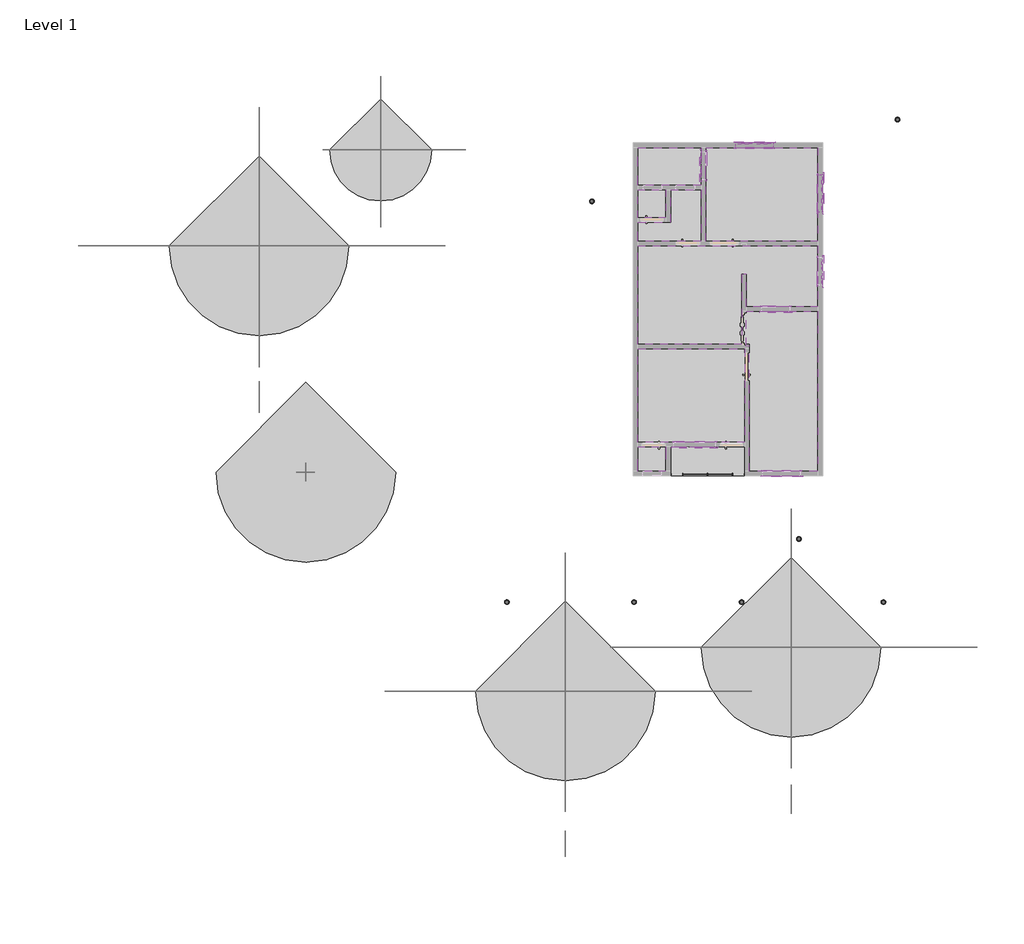
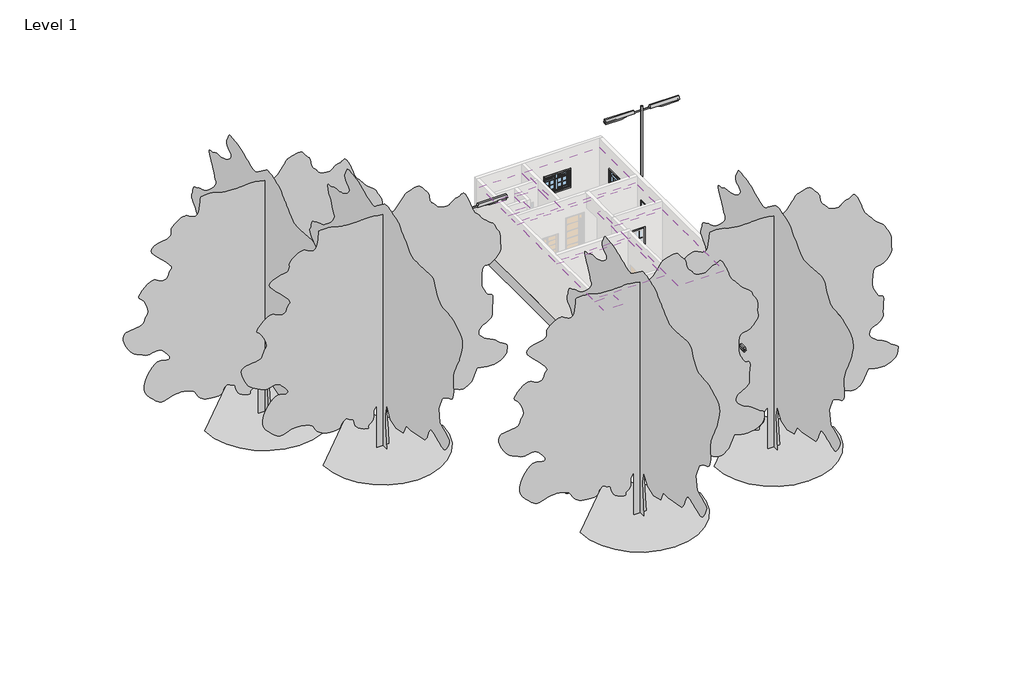
# One storey, part 2 of 2: 36 proxies, 8 coverings, 7 light fixtures, 5 geographic elements, 2 windows, 1 railing.
"""IFC4 building model written with IfcOpenShell, lengths in millimetres."""

from ifc_helpers import new_model, si_unit, point, frame, origin, place, context, project, spatial, polyline, ellipse_curve, trimmed, outline, extrude, transform, mapped, element, save
from ifc_brep_helpers import plane_surface, extruded_surface, advanced_brep
from components import m_muntin_pattern_2x2_m_muntin_pattern_2x2_ec2ff75e, m_muntin_pattern_2x2_m_muntin_pattern_2x2_6a19bea2, m_muntin_pattern_2x2_m_muntin_pattern_2x2_383df7b3, m_muntin_pattern_2x2_m_muntin_pattern_2x2_55460d9e, m_muntin_pattern_2x2_m_muntin_pattern_2x2_a9b7b7a9, m_muntin_pattern_2x2_m_muntin_pattern_2x2_c959817e, m_muntin_pattern_2x2_m_muntin_pattern_2x2_9259c5e2, m_trim_window_exterior_flat_with_sill_b1b88069, m_trim_window_exterior_flat_with_sill_8fa486dc, m_trim_window_exterior_flat_with_sill_2a9c44ae, m_trim_window_interior_flat_picture_frame_7d12f20c, m_trim_window_interior_flat_picture_frame_b6dd03a6, m_trim_window_interior_flat_picture_frame_c139440e, plinth_plinth_0a88a6c8, rpc_tree_deciduous_honey_locust_25_cc46a1f1, rpc_tree_deciduous_scarlet_oak_42_9b182cbb, light_fixture_105_street_light_dbl_105_street_light_dbl_4055396a, m_window_casement_double_awning_double_4_7efa9bbd

model = new_model("IFC4")

# Units and contexts
model_context = context("Model", 3, world=origin())
ifc_project = project(units=[si_unit("LENGTHUNIT", "METRE", prefix="MILLI")], contexts=[model_context])

# Site, building, storey
site = spatial("IfcSite", under=ifc_project)
building = spatial("IfcBuilding", under=site)
storey = spatial("IfcBuildingStorey", under=building, Name="Level 1", Elevation=0.0)

# Proxies
placement = place(None, origin())
m_muntin_pattern_2x2_m_muntin_pattern_2x2_shape = m_muntin_pattern_2x2_m_muntin_pattern_2x2_ec2ff75e(model_context)
element("IfcBuildingElementProxy", 1, Name="M_Muntin Pattern_2x2 : M_Muntin Pattern_2x2", ObjectType="M_Muntin Pattern_2x2 : M_Muntin Pattern_2x2", at=placement, inside=storey, context=model_context, shape_type="MappedRepresentation", body=[
    mapped(m_muntin_pattern_2x2_m_muntin_pattern_2x2_shape, transform((-20164.8088079, 6316.5492053, 1898.65), x_axis=(1.0, 0.0, 0.0), y_axis=(0.0, 1.0, 0.0), z_axis=(0.0, 0.0, 1.0))),
])
element("IfcBuildingElementProxy", 2, Name="M_Muntin Pattern_2x2 : M_Muntin Pattern_2x2", ObjectType="M_Muntin Pattern_2x2 : M_Muntin Pattern_2x2", at=placement, inside=storey, context=model_context, shape_type="MappedRepresentation", body=[
    mapped(m_muntin_pattern_2x2_m_muntin_pattern_2x2_shape, transform((-17648.6213079, 4984.6367053, 1898.65), x_axis=(0.0, -1.0, 0.0), y_axis=(1.0, 0.0, 0.0), z_axis=(0.0, 0.0, 1.0))),
])
element("IfcBuildingElementProxy", 3, Name="M_Muntin Pattern_2x2 : M_Muntin Pattern_2x2", ObjectType="M_Muntin Pattern_2x2 : M_Muntin Pattern_2x2", at=placement, inside=storey, context=model_context, shape_type="MappedRepresentation", body=[
    mapped(m_muntin_pattern_2x2_m_muntin_pattern_2x2_shape, transform((-18672.7572454, -4510.2007947, 1898.65), x_axis=(-1.0, 0.0, 0.0), y_axis=(0.0, -1.0, 0.0), z_axis=(0.0, 0.0, 1.0))),
])
m_muntin_pattern_2x2_m_muntin_pattern_2x2_2_shape = m_muntin_pattern_2x2_m_muntin_pattern_2x2_6a19bea2(model_context)
element("IfcBuildingElementProxy", 4, Name="M_Muntin Pattern_2x2 : M_Muntin Pattern_2x2", ObjectType="M_Muntin Pattern_2x2 : M_Muntin Pattern_2x2", at=placement, inside=storey, context=model_context, shape_type="MappedRepresentation", body=[
    mapped(m_muntin_pattern_2x2_m_muntin_pattern_2x2_2_shape, transform((-19558.3838079, 6316.5492053, 1898.65), x_axis=(-1.0, 0.0, 0.0), y_axis=(0.0, -1.0, 0.0), z_axis=(0.0, 0.0, 1.0))),
])
element("IfcBuildingElementProxy", 5, Name="M_Muntin Pattern_2x2 : M_Muntin Pattern_2x2", ObjectType="M_Muntin Pattern_2x2 : M_Muntin Pattern_2x2", at=placement, inside=storey, context=model_context, shape_type="MappedRepresentation", body=[
    mapped(m_muntin_pattern_2x2_m_muntin_pattern_2x2_2_shape, transform((-17648.6213079, 4378.2117053, 1898.65), x_axis=(0.0, 1.0, 0.0), y_axis=(-1.0, 0.0, 0.0), z_axis=(0.0, 0.0, 1.0))),
])
element("IfcBuildingElementProxy", 6, Name="M_Muntin Pattern_2x2 : M_Muntin Pattern_2x2", ObjectType="M_Muntin Pattern_2x2 : M_Muntin Pattern_2x2", at=placement, inside=storey, context=model_context, shape_type="MappedRepresentation", body=[
    mapped(m_muntin_pattern_2x2_m_muntin_pattern_2x2_2_shape, transform((-19279.1822454, -4510.2007947, 1898.65), x_axis=(1.0, 0.0, 0.0), y_axis=(0.0, 1.0, 0.0), z_axis=(0.0, 0.0, 1.0))),
])
m_muntin_pattern_2x2_m_muntin_pattern_2x2_3_shape = m_muntin_pattern_2x2_m_muntin_pattern_2x2_383df7b3(model_context)
element("IfcBuildingElementProxy", 7, Name="M_Muntin Pattern_2x2 : M_Muntin Pattern_2x2", ObjectType="M_Muntin Pattern_2x2 : M_Muntin Pattern_2x2", at=placement, inside=storey, context=model_context, shape_type="MappedRepresentation", body=[
    mapped(m_muntin_pattern_2x2_m_muntin_pattern_2x2_3_shape, transform((-19558.3838079, 6316.5492053, 2498.65), x_axis=(-1.0, 0.0, 0.0), y_axis=(0.0, -1.0, 0.0), z_axis=(0.0, 0.0, 1.0))),
])
element("IfcBuildingElementProxy", 8, Name="M_Muntin Pattern_2x2 : M_Muntin Pattern_2x2", ObjectType="M_Muntin Pattern_2x2 : M_Muntin Pattern_2x2", at=placement, inside=storey, context=model_context, shape_type="MappedRepresentation", body=[
    mapped(m_muntin_pattern_2x2_m_muntin_pattern_2x2_3_shape, transform((-20164.8088079, 6316.5492053, 2498.65), x_axis=(-1.0, 0.0, 0.0), y_axis=(0.0, -1.0, 0.0), z_axis=(0.0, 0.0, 1.0))),
])
element("IfcBuildingElementProxy", 9, Name="M_Muntin Pattern_2x2 : M_Muntin Pattern_2x2", ObjectType="M_Muntin Pattern_2x2 : M_Muntin Pattern_2x2", at=placement, inside=storey, context=model_context, shape_type="MappedRepresentation", body=[
    mapped(m_muntin_pattern_2x2_m_muntin_pattern_2x2_3_shape, transform((-17648.6213079, 4378.2117053, 2498.65), x_axis=(0.0, 1.0, 0.0), y_axis=(-1.0, 0.0, 0.0), z_axis=(0.0, 0.0, 1.0))),
])
element("IfcBuildingElementProxy", 10, Name="M_Muntin Pattern_2x2 : M_Muntin Pattern_2x2", ObjectType="M_Muntin Pattern_2x2 : M_Muntin Pattern_2x2", at=placement, inside=storey, context=model_context, shape_type="MappedRepresentation", body=[
    mapped(m_muntin_pattern_2x2_m_muntin_pattern_2x2_3_shape, transform((-17648.6213079, 4984.6367053, 2498.65), x_axis=(0.0, 1.0, 0.0), y_axis=(-1.0, 0.0, 0.0), z_axis=(0.0, 0.0, 1.0))),
])
element("IfcBuildingElementProxy", 11, Name="M_Muntin Pattern_2x2 : M_Muntin Pattern_2x2", ObjectType="M_Muntin Pattern_2x2 : M_Muntin Pattern_2x2", at=placement, inside=storey, context=model_context, shape_type="MappedRepresentation", body=[
    mapped(m_muntin_pattern_2x2_m_muntin_pattern_2x2_3_shape, transform((-19279.1822454, -4510.2007947, 2498.65), x_axis=(1.0, 0.0, 0.0), y_axis=(0.0, 1.0, 0.0), z_axis=(0.0, 0.0, 1.0))),
])
element("IfcBuildingElementProxy", 12, Name="M_Muntin Pattern_2x2 : M_Muntin Pattern_2x2", ObjectType="M_Muntin Pattern_2x2 : M_Muntin Pattern_2x2", at=placement, inside=storey, context=model_context, shape_type="MappedRepresentation", body=[
    mapped(m_muntin_pattern_2x2_m_muntin_pattern_2x2_3_shape, transform((-18672.7572454, -4510.2007947, 2498.65), x_axis=(1.0, 0.0, 0.0), y_axis=(0.0, 1.0, 0.0), z_axis=(0.0, 0.0, 1.0))),
])
m_muntin_pattern_2x2_m_muntin_pattern_2x2_4_shape = m_muntin_pattern_2x2_m_muntin_pattern_2x2_55460d9e(model_context)
element("IfcBuildingElementProxy", 13, Name="M_Muntin Pattern_2x2 : M_Muntin Pattern_2x2", ObjectType="M_Muntin Pattern_2x2 : M_Muntin Pattern_2x2", at=placement, inside=storey, context=model_context, shape_type="MappedRepresentation", body=[
    mapped(m_muntin_pattern_2x2_m_muntin_pattern_2x2_4_shape, transform((-18939.9533391, 849.1992053, 1898.65), x_axis=(-1.0, 0.0, 0.0), y_axis=(0.0, -1.0, 0.0), z_axis=(0.0, 0.0, 1.0))),
])
element("IfcBuildingElementProxy", 14, Name="M_Muntin Pattern_2x2 : M_Muntin Pattern_2x2", ObjectType="M_Muntin Pattern_2x2 : M_Muntin Pattern_2x2", at=placement, inside=storey, context=model_context, shape_type="MappedRepresentation", body=[
    mapped(m_muntin_pattern_2x2_m_muntin_pattern_2x2_4_shape, transform((-17648.6213079, 2366.8492053, 1898.65), x_axis=(0.0, -1.0, 0.0), y_axis=(1.0, 0.0, 0.0), z_axis=(0.0, 0.0, 1.0))),
])
element("IfcBuildingElementProxy", 15, Name="M_Muntin Pattern_2x2 : M_Muntin Pattern_2x2", ObjectType="M_Muntin Pattern_2x2 : M_Muntin Pattern_2x2", at=placement, inside=storey, context=model_context, shape_type="MappedRepresentation", body=[
    mapped(m_muntin_pattern_2x2_m_muntin_pattern_2x2_4_shape, transform((-21591.9713079, 5362.4617053, 1898.65), x_axis=(0.0, 1.0, 0.0), y_axis=(-1.0, 0.0, 0.0), z_axis=(0.0, 0.0, 1.0))),
])
m_muntin_pattern_2x2_m_muntin_pattern_2x2_5_shape = m_muntin_pattern_2x2_m_muntin_pattern_2x2_a9b7b7a9(model_context)
element("IfcBuildingElementProxy", 16, Name="M_Muntin Pattern_2x2 : M_Muntin Pattern_2x2", ObjectType="M_Muntin Pattern_2x2 : M_Muntin Pattern_2x2", at=placement, inside=storey, context=model_context, shape_type="MappedRepresentation", body=[
    mapped(m_muntin_pattern_2x2_m_muntin_pattern_2x2_5_shape, transform((-19393.9783391, 849.1992053, 1898.65), x_axis=(1.0, 0.0, 0.0), y_axis=(0.0, 1.0, 0.0), z_axis=(0.0, 0.0, 1.0))),
])
element("IfcBuildingElementProxy", 17, Name="M_Muntin Pattern_2x2 : M_Muntin Pattern_2x2", ObjectType="M_Muntin Pattern_2x2 : M_Muntin Pattern_2x2", at=placement, inside=storey, context=model_context, shape_type="MappedRepresentation", body=[
    mapped(m_muntin_pattern_2x2_m_muntin_pattern_2x2_5_shape, transform((-17648.6213079, 1912.8242053, 1898.65), x_axis=(0.0, 1.0, 0.0), y_axis=(-1.0, 0.0, 0.0), z_axis=(0.0, 0.0, 1.0))),
])
element("IfcBuildingElementProxy", 18, Name="M_Muntin Pattern_2x2 : M_Muntin Pattern_2x2", ObjectType="M_Muntin Pattern_2x2 : M_Muntin Pattern_2x2", at=placement, inside=storey, context=model_context, shape_type="MappedRepresentation", body=[
    mapped(m_muntin_pattern_2x2_m_muntin_pattern_2x2_5_shape, transform((-21591.9713079, 5816.4867053, 1898.65), x_axis=(0.0, -1.0, 0.0), y_axis=(1.0, 0.0, 0.0), z_axis=(0.0, 0.0, 1.0))),
])
m_muntin_pattern_2x2_m_muntin_pattern_2x2_6_shape = m_muntin_pattern_2x2_m_muntin_pattern_2x2_c959817e(model_context)
element("IfcBuildingElementProxy", 19, Name="M_Muntin Pattern_2x2 : M_Muntin Pattern_2x2", ObjectType="M_Muntin Pattern_2x2 : M_Muntin Pattern_2x2", at=placement, inside=storey, context=model_context, shape_type="MappedRepresentation", body=[
    mapped(m_muntin_pattern_2x2_m_muntin_pattern_2x2_6_shape, transform((-21364.4296412, -3570.4007947, 1898.65), x_axis=(-1.0, 0.0, 0.0), y_axis=(0.0, -1.0, 0.0), z_axis=(0.0, 0.0, 1.0))),
])
m_muntin_pattern_2x2_m_muntin_pattern_2x2_7_shape = m_muntin_pattern_2x2_m_muntin_pattern_2x2_9259c5e2(model_context)
element("IfcBuildingElementProxy", 20, Name="M_Muntin Pattern_2x2 : M_Muntin Pattern_2x2", ObjectType="M_Muntin Pattern_2x2 : M_Muntin Pattern_2x2", at=placement, inside=storey, context=model_context, shape_type="MappedRepresentation", body=[
    mapped(m_muntin_pattern_2x2_m_muntin_pattern_2x2_7_shape, transform((-22257.6629746, -3570.4007947, 1898.65), x_axis=(1.0, 0.0, 0.0), y_axis=(0.0, 1.0, 0.0), z_axis=(0.0, 0.0, 1.0))),
])
element("IfcBuildingElementProxy", 21, Name="M_Muntin Pattern_2x2 : M_Muntin Pattern_2x2", ObjectType="M_Muntin Pattern_2x2 : M_Muntin Pattern_2x2", at=placement, inside=storey, context=model_context, shape_type="MappedRepresentation", body=[
    mapped(m_muntin_pattern_2x2_m_muntin_pattern_2x2_7_shape, transform((-21811.0463079, -3570.4007947, 1898.65), x_axis=(1.0, 0.0, 0.0), y_axis=(0.0, 1.0, 0.0), z_axis=(0.0, 0.0, 1.0))),
])
m_trim_window_exterior_flat_with_sill_shape = m_trim_window_exterior_flat_with_sill_b1b88069(model_context)
element("IfcBuildingElementProxy", 22, Name="M_Trim-Window-Exterior-Flat : with Sill", ObjectType="M_Trim-Window-Exterior-Flat : with Sill", at=placement, inside=storey, context=model_context, shape_type="MappedRepresentation", body=[
    mapped(m_trim_window_exterior_flat_with_sill_shape, transform((-19861.5963079, 6326.0742053, 2728.8), x_axis=(-1.0, 0.0, 0.0), y_axis=(0.0, 0.0, 1.0), z_axis=(0.0, 1.0, 0.0))),
])
element("IfcBuildingElementProxy", 23, Name="M_Trim-Window-Exterior-Flat : with Sill", ObjectType="M_Trim-Window-Exterior-Flat : with Sill", at=placement, inside=storey, context=model_context, shape_type="MappedRepresentation", body=[
    mapped(m_trim_window_exterior_flat_with_sill_shape, transform((-17639.0963079, 4681.4242053, 2728.8), x_axis=(0.0, 1.0, 0.0), y_axis=(0.0, 0.0, 1.0), z_axis=(1.0, 0.0, 0.0))),
])
element("IfcBuildingElementProxy", 24, Name="M_Trim-Window-Exterior-Flat : with Sill", ObjectType="M_Trim-Window-Exterior-Flat : with Sill", at=placement, inside=storey, context=model_context, shape_type="MappedRepresentation", body=[
    mapped(m_trim_window_exterior_flat_with_sill_shape, transform((-18975.9697454, -4519.7257947, 2728.8), x_axis=(1.0, 0.0, 0.0), y_axis=(0.0, 0.0, 1.0), z_axis=(0.0, -1.0, 0.0))),
])
m_trim_window_exterior_flat_with_sill_2_shape = m_trim_window_exterior_flat_with_sill_8fa486dc(model_context)
element("IfcBuildingElementProxy", 25, Name="M_Trim-Window-Exterior-Flat : with Sill", ObjectType="M_Trim-Window-Exterior-Flat : with Sill", at=placement, inside=storey, context=model_context, shape_type="MappedRepresentation", body=[
    mapped(m_trim_window_exterior_flat_with_sill_2_shape, transform((-19166.9658391, 839.6742053, 2728.8), x_axis=(1.0, 0.0, 0.0), y_axis=(0.0, 0.0, 1.0), z_axis=(0.0, -1.0, 0.0))),
])
element("IfcBuildingElementProxy", 26, Name="M_Trim-Window-Exterior-Flat : with Sill", ObjectType="M_Trim-Window-Exterior-Flat : with Sill", at=placement, inside=storey, context=model_context, shape_type="MappedRepresentation", body=[
    mapped(m_trim_window_exterior_flat_with_sill_2_shape, transform((-17639.0963079, 2139.8367053, 2728.8), x_axis=(0.0, 1.0, 0.0), y_axis=(0.0, 0.0, 1.0), z_axis=(1.0, 0.0, 0.0))),
])
element("IfcBuildingElementProxy", 27, Name="M_Trim-Window-Exterior-Flat : with Sill", ObjectType="M_Trim-Window-Exterior-Flat : with Sill", at=placement, inside=storey, context=model_context, shape_type="MappedRepresentation", body=[
    mapped(m_trim_window_exterior_flat_with_sill_2_shape, transform((-21601.4963079, 5589.4742053, 2728.8), x_axis=(0.0, -1.0, 0.0), y_axis=(0.0, 0.0, 1.0), z_axis=(-1.0, 0.0, 0.0))),
])
m_trim_window_exterior_flat_with_sill_3_shape = m_trim_window_exterior_flat_with_sill_2a9c44ae(model_context)
element("IfcBuildingElementProxy", 28, Name="M_Trim-Window-Exterior-Flat : with Sill", ObjectType="M_Trim-Window-Exterior-Flat : with Sill", at=placement, inside=storey, context=model_context, shape_type="MappedRepresentation", body=[
    mapped(m_trim_window_exterior_flat_with_sill_3_shape, transform((-21811.0463079, -3579.9257947, 2628.8), x_axis=(1.0, 0.0, 0.0), y_axis=(0.0, 0.0, 1.0), z_axis=(0.0, -1.0, 0.0))),
])
m_trim_window_interior_flat_picture_frame_shape = m_trim_window_interior_flat_picture_frame_7d12f20c(model_context)
element("IfcBuildingElementProxy", 29, Name="M_Trim-Window-Interior-Flat : Picture Frame", ObjectType="M_Trim-Window-Interior-Flat : Picture Frame", at=placement, inside=storey, context=model_context, shape_type="MappedRepresentation", body=[
    mapped(m_trim_window_interior_flat_picture_frame_shape, transform((-19861.5963079, 6173.6742053, 2728.8), x_axis=(1.0, 0.0, 0.0), y_axis=(0.0, 0.0, 1.0), z_axis=(0.0, -1.0, 0.0))),
])
element("IfcBuildingElementProxy", 30, Name="M_Trim-Window-Interior-Flat : Picture Frame", ObjectType="M_Trim-Window-Interior-Flat : Picture Frame", at=placement, inside=storey, context=model_context, shape_type="MappedRepresentation", body=[
    mapped(m_trim_window_interior_flat_picture_frame_shape, transform((-17791.4963079, 4681.4242053, 2728.8), x_axis=(0.0, -1.0, 0.0), y_axis=(0.0, 0.0, 1.0), z_axis=(-1.0, 0.0, 0.0))),
])
element("IfcBuildingElementProxy", 31, Name="M_Trim-Window-Interior-Flat : Picture Frame", ObjectType="M_Trim-Window-Interior-Flat : Picture Frame", at=placement, inside=storey, context=model_context, shape_type="MappedRepresentation", body=[
    mapped(m_trim_window_interior_flat_picture_frame_shape, transform((-18975.9697454, -4367.3257947, 2728.8), x_axis=(-1.0, 0.0, 0.0), y_axis=(0.0, 0.0, 1.0), z_axis=(0.0, 1.0, 0.0))),
])
m_trim_window_interior_flat_picture_frame_2_shape = m_trim_window_interior_flat_picture_frame_b6dd03a6(model_context)
element("IfcBuildingElementProxy", 32, Name="M_Trim-Window-Interior-Flat : Picture Frame", ObjectType="M_Trim-Window-Interior-Flat : Picture Frame", at=placement, inside=storey, context=model_context, shape_type="MappedRepresentation", body=[
    mapped(m_trim_window_interior_flat_picture_frame_2_shape, transform((-19166.9658391, 992.0742053, 2728.8), x_axis=(-1.0, 0.0, 0.0), y_axis=(0.0, 0.0, 1.0), z_axis=(0.0, 1.0, 0.0))),
])
element("IfcBuildingElementProxy", 33, Name="M_Trim-Window-Interior-Flat : Picture Frame", ObjectType="M_Trim-Window-Interior-Flat : Picture Frame", at=placement, inside=storey, context=model_context, shape_type="MappedRepresentation", body=[
    mapped(m_trim_window_interior_flat_picture_frame_2_shape, transform((-17791.4963079, 2139.8367053, 2728.8), x_axis=(0.0, -1.0, 0.0), y_axis=(0.0, 0.0, 1.0), z_axis=(-1.0, 0.0, 0.0))),
])
element("IfcBuildingElementProxy", 34, Name="M_Trim-Window-Interior-Flat : Picture Frame", ObjectType="M_Trim-Window-Interior-Flat : Picture Frame", at=placement, inside=storey, context=model_context, shape_type="MappedRepresentation", body=[
    mapped(m_trim_window_interior_flat_picture_frame_2_shape, transform((-21449.0963079, 5589.4742053, 2728.8), x_axis=(0.0, 1.0, 0.0), y_axis=(0.0, 0.0, 1.0), z_axis=(1.0, 0.0, 0.0))),
])
m_trim_window_interior_flat_picture_frame_3_shape = m_trim_window_interior_flat_picture_frame_c139440e(model_context)
element("IfcBuildingElementProxy", 35, Name="M_Trim-Window-Interior-Flat : Picture Frame", ObjectType="M_Trim-Window-Interior-Flat : Picture Frame", at=placement, inside=storey, context=model_context, shape_type="MappedRepresentation", body=[
    mapped(m_trim_window_interior_flat_picture_frame_3_shape, transform((-21811.0463079, -3427.5257947, 2628.8), x_axis=(-1.0, 0.0, 0.0), y_axis=(0.0, 0.0, 1.0), z_axis=(0.0, 1.0, 0.0))),
])
plinth_plinth_shape = plinth_plinth_0a88a6c8(model_context)
element("IfcBuildingElementProxy", 36, Name="PLINTH : PLINTH", ObjectType="PLINTH : PLINTH", at=placement, inside=storey, context=model_context, shape_type="MappedRepresentation", body=[
    mapped(plinth_plinth_shape, transform((0.0, 0.0, 0.0), x_axis=(1.0, 0.0, 0.0), y_axis=(0.0, 1.0, 0.0), z_axis=(0.0, 0.0, 1.0))),
])

# Coverings
element("IfcCovering", 37, ObjectType="2' x 4' ACT System", at=placement, inside=storey, context=model_context, shape_type="SweptSolid", body=[
    extrude(outline(polyline([(-23658.8963079, 6173.6742053), (-21601.4963079, 6173.6742053), (-21601.4963079, 4954.4742053), (-23658.8963079, 4954.4742053), (-23658.8963079, 6173.6742053)])), frame((0.0, 0.0, 3352.8), z_axis=(0.0, 0.0, 1.0), x_axis=(1.0, 0.0, 0.0)), (0.0, 0.0, 1.0), 57.15),
])
element("IfcCovering", 38, ObjectType="2' x 4' ACT System", at=placement, inside=storey, context=model_context, shape_type="SweptSolid", body=[
    extrude(outline(polyline([(-21449.0963079, 3125.6742053), (-21449.0963079, 6173.6742053), (-17791.4963079, 6173.6742053), (-17791.4963079, 3125.6742053), (-21449.0963079, 3125.6742053)])), frame((0.0, 0.0, 3352.8), z_axis=(0.0, 0.0, 1.0), x_axis=(1.0, 0.0, 0.0)), (0.0, 0.0, 1.0), 57.15),
])
element("IfcCovering", 39, ObjectType="2' x 4' ACT System", at=placement, inside=storey, context=model_context, shape_type="SweptSolid", body=[
    extrude(outline(polyline([(-21601.4963079, 3125.6742053), (-23658.8963079, 3125.6742053), (-23658.8963079, 3735.2742053), (-22592.0963079, 3735.2742053), (-22592.0963079, 4802.0742053), (-21601.4963079, 4802.0742053), (-21601.4963079, 3125.6742053)])), frame((0.0, 0.0, 3352.8), z_axis=(0.0, 0.0, 1.0), x_axis=(1.0, 0.0, 0.0)), (0.0, 0.0, 1.0), 57.15),
])
element("IfcCovering", 40, ObjectType="2' x 4' ACT System", at=placement, inside=storey, context=model_context, shape_type="SweptSolid", body=[
    extrude(outline(polyline([(-22744.4963079, 3887.6742053), (-23658.8963079, 3887.6742053), (-23658.8963079, 4802.0742053), (-22744.4963079, 4802.0742053), (-22744.4963079, 3887.6742053)])), frame((0.0, 0.0, 3352.8), z_axis=(0.0, 0.0, 1.0), x_axis=(1.0, 0.0, 0.0)), (0.0, 0.0, 1.0), 57.15),
])
element("IfcCovering", 41, ObjectType="2' x 4' ACT System", at=placement, inside=storey, context=model_context, shape_type="SweptSolid", body=[
    extrude(outline(polyline([(-17791.4963079, 2973.2742053), (-17791.4963079, 992.0742053), (-20128.2963079, 992.0742053), (-20128.2963079, 2050.5574639), (-20280.6963079, 2050.5574639), (-20280.6963079, 915.8742053), (-20280.6963079, -227.1257947), (-23658.8963079, -227.1257947), (-23658.8963079, 2973.2742053), (-17791.4963079, 2973.2742053)])), frame((0.0, 0.0, 3352.8), z_axis=(0.0, 0.0, 1.0), x_axis=(1.0, 0.0, 0.0)), (0.0, 0.0, 1.0), 57.15),
])
element("IfcCovering", 42, ObjectType="2' x 4' ACT System", at=placement, inside=storey, context=model_context, shape_type="SweptSolid", body=[
    extrude(outline(polyline([(-20179.0963079, -3427.5257947), (-23658.8963079, -3427.5257947), (-23658.8963079, -379.5257947), (-20179.0963079, -379.5257947), (-20179.0963079, -3427.5257947)])), frame((0.0, 0.0, 3352.8), z_axis=(0.0, 0.0, 1.0), x_axis=(1.0, 0.0, 0.0)), (0.0, 0.0, 1.0), 57.15),
])
element("IfcCovering", 43, ObjectType="2' x 4' ACT System", at=placement, inside=storey, context=model_context, shape_type="SweptSolid", body=[
    extrude(outline(polyline([(-17791.4963079, 839.6742053), (-17791.4963079, -4367.3257947), (-20026.6963079, -4367.3257947), (-20026.6963079, -303.3257947), (-20128.2963079, -303.3257947), (-20128.2963079, 839.6742053), (-17791.4963079, 839.6742053)])), frame((0.0, 0.0, 3352.8), z_axis=(0.0, 0.0, 1.0), x_axis=(1.0, 0.0, 0.0)), (0.0, 0.0, 1.0), 57.15),
])
element("IfcCovering", 44, ObjectType="2' x 4' ACT System", at=placement, inside=storey, context=model_context, shape_type="SweptSolid", body=[
    extrude(outline(polyline([(-22744.4963079, -4367.3257947), (-23658.8963079, -4367.3257947), (-23658.8963079, -3579.9257947), (-22744.4963079, -3579.9257947), (-22744.4963079, -4367.3257947)])), frame((0.0, 0.0, 3352.8), z_axis=(0.0, 0.0, 1.0), x_axis=(1.0, 0.0, 0.0)), (0.0, 0.0, 1.0), 57.15),
])

# Geographic elements
rpc_tree_deciduous_honey_locust_25_shape = rpc_tree_deciduous_honey_locust_25_cc46a1f1(model_context)
element("IfcGeographicElement", 45, ObjectType="RPC Tree - Deciduous : Honey Locust - 25'", at=placement, inside=storey, context=model_context, shape_type="MappedRepresentation", body=[
    mapped(rpc_tree_deciduous_honey_locust_25_shape, transform((-32040.8963079, 6097.4742053, -1981.2), x_axis=(1.0, 0.0, 0.0), y_axis=(0.0, 1.0, 0.0), z_axis=(0.0, 0.0, 1.0))),
])
rpc_tree_deciduous_scarlet_oak_42_shape = rpc_tree_deciduous_scarlet_oak_42_9b182cbb(model_context)
element("IfcGeographicElement", 46, ObjectType="RPC Tree - Deciduous : Scarlet Oak - 42'", at=placement, inside=storey, context=model_context, shape_type="MappedRepresentation", body=[
    mapped(rpc_tree_deciduous_scarlet_oak_42_shape, transform((-36003.2963079, 2973.2742053, -1981.2), x_axis=(1.0, 0.0, 0.0), y_axis=(0.0, 1.0, 0.0), z_axis=(0.0, 0.0, 1.0))),
])
element("IfcGeographicElement", 47, ObjectType="RPC Tree - Deciduous : Scarlet Oak - 42'", at=placement, inside=storey, context=model_context, shape_type="MappedRepresentation", body=[
    mapped(rpc_tree_deciduous_scarlet_oak_42_shape, transform((-26020.9810533, -11530.6777483, -1928.1661647), x_axis=(1.0, 0.0, 0.0), y_axis=(0.0, 1.0, 0.0), z_axis=(0.0, 0.0, 1.0))),
])
element("IfcGeographicElement", 48, ObjectType="RPC Tree - Deciduous : Scarlet Oak - 42'", at=placement, inside=storey, context=model_context, shape_type="MappedRepresentation", body=[
    mapped(rpc_tree_deciduous_scarlet_oak_42_shape, transform((-18667.7963079, -10107.7142603, -1960.082478), x_axis=(1.0, 0.0, 0.0), y_axis=(0.0, 1.0, 0.0), z_axis=(0.0, 0.0, 1.0))),
])
element("IfcGeographicElement", 49, ObjectType="RPC Tree - Deciduous : Scarlet Oak - 42'", at=placement, inside=storey, context=model_context, shape_type="MappedRepresentation", body=[
    mapped(rpc_tree_deciduous_scarlet_oak_42_shape, transform((-34477.6655413, -4403.0556437, 186.7246553), x_axis=(1.0, 0.0, 0.0), y_axis=(0.0, 1.0, 0.0), z_axis=(0.0, 0.0, 1.0))),
])

# Light fixtures
light_fixture_105_street_light_dbl_105_street_light_dbl_shape = light_fixture_105_street_light_dbl_105_street_light_dbl_4055396a(model_context)
element("IfcLightFixture", 50, ObjectType="105_Street Light - Dbl : 105_Street Light - Dbl", at=placement, inside=storey, context=model_context, shape_type="MappedRepresentation", body=[
    mapped(light_fixture_105_street_light_dbl_105_street_light_dbl_shape, transform((-25157.4963079, 4377.509477, -1981.2), x_axis=(0.0, 1.0, 0.0), y_axis=(-1.0, 0.0, 0.0), z_axis=(0.0, 0.0, 1.0))),
])
element("IfcLightFixture", 51, ObjectType="105_Street Light - Dbl : 105_Street Light - Dbl", at=placement, inside=storey, context=model_context, shape_type="MappedRepresentation", body=[
    mapped(light_fixture_105_street_light_dbl_105_street_light_dbl_shape, transform((-15200.6963079, 7044.509477, -1981.2), x_axis=(0.0, 1.0, 0.0), y_axis=(-1.0, 0.0, 0.0), z_axis=(0.0, 0.0, 1.0))),
])
element("IfcLightFixture", 52, ObjectType="105_Street Light - Dbl : 105_Street Light - Dbl", at=placement, inside=storey, context=model_context, shape_type="MappedRepresentation", body=[
    mapped(light_fixture_105_street_light_dbl_105_street_light_dbl_shape, transform((-18457.3610362, -6577.1257947, -1981.2), x_axis=(1.0, 0.0, 0.0), y_axis=(0.0, 1.0, 0.0), z_axis=(0.0, 0.0, 1.0))),
])
element("IfcLightFixture", 53, ObjectType="105_Street Light - Dbl : 105_Street Light - Dbl", at=placement, inside=storey, context=model_context, shape_type="MappedRepresentation", body=[
    mapped(light_fixture_105_street_light_dbl_105_street_light_dbl_shape, transform((-27969.6610362, -8634.5257947, -1981.2), x_axis=(1.0, 0.0, 0.0), y_axis=(0.0, 1.0, 0.0), z_axis=(0.0, 0.0, 1.0))),
])
element("IfcLightFixture", 54, ObjectType="105_Street Light - Dbl : 105_Street Light - Dbl", at=placement, inside=storey, context=model_context, shape_type="MappedRepresentation", body=[
    mapped(light_fixture_105_street_light_dbl_105_street_light_dbl_shape, transform((-23829.4610362, -8634.5257947, -1981.2), x_axis=(1.0, 0.0, 0.0), y_axis=(0.0, 1.0, 0.0), z_axis=(0.0, 0.0, 1.0))),
])
element("IfcLightFixture", 55, ObjectType="105_Street Light - Dbl : 105_Street Light - Dbl", at=placement, inside=storey, context=model_context, shape_type="MappedRepresentation", body=[
    mapped(light_fixture_105_street_light_dbl_105_street_light_dbl_shape, transform((-20324.2610362, -8634.5257947, -1981.2), x_axis=(1.0, 0.0, 0.0), y_axis=(0.0, 1.0, 0.0), z_axis=(0.0, 0.0, 1.0))),
])
element("IfcLightFixture", 56, ObjectType="105_Street Light - Dbl : 105_Street Light - Dbl", at=placement, inside=storey, context=model_context, shape_type="MappedRepresentation", body=[
    mapped(light_fixture_105_street_light_dbl_105_street_light_dbl_shape, transform((-15701.4610362, -8634.5257947, -1981.2), x_axis=(1.0, 0.0, 0.0), y_axis=(0.0, 1.0, 0.0), z_axis=(0.0, 0.0, 1.0))),
])

# Railing
element("IfcRailing", 57, ObjectType="Glass Panel - Bottom Fill", at=placement, inside=storey, context=model_context, shape_type="SolidModel", body=[
    advanced_brep(
    [(-22592.0963079, -4430.8257947, 1828.8), (-22592.0963079, -4507.0257947, 1828.8), (-20179.0963079, -4430.8257947, 1828.8), (-20179.0963079, -4507.0257947, 1828.8)],
    [
        (0, 1, ellipse_curve(frame((-22592.0963079, -4468.9257947, 1828.8), z_axis=(-1.0, 0.0, 0.0), x_axis=(0.0, -1.0, 0.0)), 38.1, 28.575)),
        (1, 0, ellipse_curve(frame((-22592.0963079, -4468.9257947, 1828.8), z_axis=(-1.0, 0.0, 0.0), x_axis=(0.0, -1.0, 0.0)), 38.1, 28.575)),
        (2, 3, ellipse_curve(frame((-20179.0963079, -4468.9257947, 1828.8), z_axis=(1.0, 0.0, 0.0), x_axis=(0.0, -1.0, 0.0)), 38.1, 28.575)),
        (3, 2, ellipse_curve(frame((-20179.0963079, -4468.9257947, 1828.8), z_axis=(1.0, 0.0, 0.0), x_axis=(0.0, -1.0, 0.0)), 38.1, 28.575)),
        (0, 2),
        (3, 1),
    ],
    [
        plane_surface(frame((-22592.0963079, -4468.9257947, 1828.8), z_axis=(-1.0, 0.0, 0.0), x_axis=(0.0, 1.0, 0.0))),
        plane_surface(frame((-20179.0963079, -4468.9257947, 1828.8), z_axis=(1.0, 0.0, 0.0), x_axis=(0.0, 1.0, 0.0))),
        extruded_surface(trimmed(ellipse_curve(frame((-20179.0963079, -4468.9257947, 1828.8), z_axis=(-1.0, 0.0, 0.0), x_axis=(0.0, -1.0, 0.0)), 38.1, 28.575), [point((-20179.0963079, -4430.8257947, 1828.8))], [point((-20179.0963079, -4507.0257947, 1828.8))], True, "CARTESIAN"), (-2413.0, 0.0, 0.0), 2413.0),
        extruded_surface(trimmed(ellipse_curve(frame((-20179.0963079, -4468.9257947, 1828.8), z_axis=(-1.0, 0.0, 0.0), x_axis=(0.0, -1.0, 0.0)), 38.1, 28.575), [point((-20179.0963079, -4507.0257947, 1828.8))], [point((-20179.0963079, -4430.8257947, 1828.8))], True, "CARTESIAN"), (-2413.0, 0.0, 0.0), 2413.0),
    ],
    [
        (0, [[1, 2]]),
        (1, [[3, 4]]),
        (2, [[-1, 5, -4, 6]]),
        (3, [[-2, -6, -3, -5]]),
    ],
),
    extrude(outline(polyline([(-22592.0963079, -4481.6257947), (-22592.0963079, -4456.2257947), (-20179.0963079, -4456.2257947), (-20179.0963079, -4481.6257947), (-22592.0963079, -4481.6257947)])), frame((0.0, 0.0, 1511.3), z_axis=(0.0, 0.0, 1.0), x_axis=(1.0, 0.0, 0.0)), (0.0, 0.0, 1.0), 25.4),
    extrude(outline(polyline([(-22592.0963079, -4481.6257947), (-22592.0963079, -4456.2257947), (-20179.0963079, -4456.2257947), (-20179.0963079, -4481.6257947), (-22592.0963079, -4481.6257947)])), frame((0.0, 0.0, 1308.1), z_axis=(0.0, 0.0, 1.0), x_axis=(1.0, 0.0, 0.0)), (0.0, 0.0, 1.0), 25.4),
    extrude(outline(polyline([(-20579.1463079, -4494.3257947), (-20579.1463079, -4443.5257947), (-20566.4463079, -4443.5257947), (-20566.4463079, -4494.3257947), (-20579.1463079, -4494.3257947)])), frame((0.0, 0.0, 609.6), z_axis=(0.0, 0.0, 1.0), x_axis=(1.0, 0.0, 0.0)), (0.0, 0.0, 1.0), 1190.625),
    extrude(outline(polyline([(-21385.5963079, -4462.3906377), (-20572.7963079, -4462.3906377), (-20572.7963079, -4468.7406377), (-21385.5963079, -4468.7406377), (-21385.5963079, -4462.3906377)])), frame((0.0, 0.0, 711.2), z_axis=(0.0, 0.0, 1.0), x_axis=(1.0, 0.0, 0.0)), (0.0, 0.0, 1.0), 711.2),
    extrude(outline(polyline([(-21391.9463079, -4494.3257947), (-21391.9463079, -4443.5257947), (-21379.2463079, -4443.5257947), (-21379.2463079, -4494.3257947), (-21391.9463079, -4494.3257947)])), frame((0.0, 0.0, 609.6), z_axis=(0.0, 0.0, 1.0), x_axis=(1.0, 0.0, 0.0)), (0.0, 0.0, 1.0), 1190.625),
    extrude(outline(polyline([(-22198.3963079, -4462.3906377), (-21385.5963079, -4462.3906377), (-21385.5963079, -4468.7406377), (-22198.3963079, -4468.7406377), (-22198.3963079, -4462.3906377)])), frame((0.0, 0.0, 711.2), z_axis=(0.0, 0.0, 1.0), x_axis=(1.0, 0.0, 0.0)), (0.0, 0.0, 1.0), 711.2),
    extrude(outline(polyline([(-22204.7463079, -4494.3257947), (-22204.7463079, -4443.5257947), (-22192.0463079, -4443.5257947), (-22192.0463079, -4494.3257947), (-22204.7463079, -4494.3257947)])), frame((0.0, 0.0, 609.6), z_axis=(0.0, 0.0, 1.0), x_axis=(1.0, 0.0, 0.0)), (0.0, 0.0, 1.0), 1190.625),
    extrude(outline(polyline([(-20191.7963079, -4478.4507947), (-20191.7963079, -4459.4007947), (-20172.7463079, -4459.4007947), (-20172.7463079, -4478.4507947), (-20191.7963079, -4478.4507947)])), frame((0.0, 0.0, 609.6), z_axis=(0.0, 0.0, 1.0), x_axis=(1.0, 0.0, 0.0)), (0.0, 0.0, 1.0), 1190.625),
    extrude(outline(polyline([(-22598.4463079, -4478.4507947), (-22598.4463079, -4459.4007947), (-22579.3963079, -4459.4007947), (-22579.3963079, -4478.4507947), (-22598.4463079, -4478.4507947)])), frame((0.0, 0.0, 609.6), z_axis=(0.0, 0.0, 1.0), x_axis=(1.0, 0.0, 0.0)), (0.0, 0.0, 1.0), 1190.625),
])

# Windows
m_window_casement_double_awning_double_4_shape = m_window_casement_double_awning_double_4_7efa9bbd(model_context)
element("IfcWindow", 58, ObjectType="M_Window-Casement-Double-Awning-Double : 4'", at=placement, inside=storey, context=model_context, shape_type="MappedRepresentation", body=[
    mapped(m_window_casement_double_awning_double_4_shape, transform((-19861.5963079, 6249.8742053, 928.8), x_axis=(1.0, 0.0, 0.0), y_axis=(0.0, 1.0, 0.0), z_axis=(0.0, 0.0, 1.0))),
])
element("IfcWindow", 59, ObjectType="M_Window-Casement-Double-Awning-Double : 4'", at=placement, inside=storey, context=model_context, shape_type="MappedRepresentation", body=[
    mapped(m_window_casement_double_awning_double_4_shape, transform((-17715.2963079, 4681.4242053, 928.8), x_axis=(0.0, -1.0, 0.0), y_axis=(1.0, 0.0, 0.0), z_axis=(0.0, 0.0, 1.0))),
])

save(model, "model.ifc")

# Revit data of these elements
# Type "M_Muntin Pattern_2x2 : M_Muntin Pattern_2x2"
#   Width [instance default] = 3' - 11.24409"
#   Thickness = 0' - 0 1/2"
#   Height [instance default] = 3' - 11.24409"
#   Distance = 0' - 0 3/4"
#   Interior Material [instance default] = none
#   Exterior Material [instance default] = none
#   Default Elevation = 0
# Type "M_Trim-Window-Exterior-Flat : with Sill"
#   Trim Width = 0' - 2.3622"
#   Trim Thickness_Picture Frame = 0' - 1.1811"
#   Trim Thickness_with Sill = 0' - 0 3/4"
#   Sill Thickness = 0' - 1.1811"
#   Opening Width [instance default] = 1' - 11.62205"
#   Opening Height [instance default] = 2' - 11.43307"
#   Default Elevation = 3' - 11.24409"
#   Sill = yes
#   Picture Frame = no
#   Trim Material [instance default] = none
# Type "M_Trim-Window-Interior-Flat : Picture Frame"
#   Trim Thickness_Picture Frame = 0' - 1.1811"
#   Trim Width = 0' - 2.3622"
#   Trim Thickness_with Sill = 0' - 0.7874"
#   Sill Thickness = 0' - 1.1811"
#   Opening Width [instance default] = 1' - 11.62205"
#   Opening Height [instance default] = 2' - 11.43307"
#   Default Elevation = 3' - 11.24409"
#   Sill = no
#   Picture Frame = yes
#   Trim Material [instance default] = none
# Type "2' x 4' ACT System"
#   Assembly Code = "C3030210"
#   built-in parameter 1002203 = 1 (stored number, unit not read)
#   built-in parameter 1002202 = 1 (stored number, unit not read)
#   Layers, outside or top first: 0' - 1 5/8" "Default" (function 1); 0' - 0 5/8" "Acoustic Ceiling Tile 24 x 48" (function 5)
# Type "RPC Tree - Deciduous : Honey Locust - 25'"
#   built-in parameter 1005198 = "{2, 15},{39, RPC-16-G2VH-N100-5X50-0000-ST1L-LVER-AU},{1, 0},{1, 0},{2, 13},{1, 8},{5, Color},{1, 0},{1, 0},{3, 0.8},{3, 0.8},{3, 0.8},{1, 8},{7, BBoxMin},{1, 0},{1, 0},{1, 0},{1, 0},{1, 0},{1, 8},{7, BBoxMax},{1, 0},{1, 0},{1, 0},{1, 0},{1, 0},{2, 11},{9, RPCTypeId},{1, 0},{1, 0},{39, RPC-16-G2VH-N100-5X50-0000-ST1L-LVER-AU},{1, 6},{14, RPCPlantHeight},{1, 0},{1, 0},{2, 25},{2, 11},{7, keyword},{1, 0},{1, 0},{34, :RPCs:Trees [General]:Geometry:RPC},{2, 11},{8, category},{1, 0},{1, 0},{15, Trees [General]},{2, 11},{12, LocalizedUID},{1, 0},{1, 0},{12, Honey-Locust},{2, 14},{6, Height},{1, 0},{1, 0},{2, 25},{1, 2},{16, Cast Reflections},{1, 0},{1, 0},{1, 0},{1, 2},{12, Cast Shadows},{1, 0},{1, 0},{1, 1},{1, 2},{9, Lock View},{1, 0},{1, 0},{1, 0},{1, 4},{5, ViewC},{1, 0},{1, 0},{1, 0},{21, assetlibrary_base.fbx},{1, 5},"
#   built-in parameter 1005195 = "RPC-16-G2VH-N100-5X50-0000-ST1L-LVER-AU"
#   Type Comments = "Honey Locust"
#   Assembly Code = "G2050500"
#   Height = 25' - 0"
#   Default Elevation = 0
# Type "RPC Tree - Deciduous : Scarlet Oak - 42'"
#   built-in parameter 1005198 = "{2, 15},{39, RPC-16-G0FB-J5PX-0LX6-U000-ST1L-LVER-AU},{1, 0},{1, 0},{2, 13},{1, 8},{5, Color},{1, 0},{1, 0},{3, 0.8},{3, 0.8},{3, 0.8},{1, 8},{7, BBoxMin},{1, 0},{1, 0},{1, 0},{1, 0},{1, 0},{1, 8},{7, BBoxMax},{1, 0},{1, 0},{1, 0},{1, 0},{1, 0},{2, 11},{9, RPCTypeId},{1, 0},{1, 0},{39, RPC-16-G0FB-J5PX-0LX6-U000-ST1L-LVER-AU},{1, 6},{14, RPCPlantHeight},{1, 0},{1, 0},{2, 42},{2, 11},{7, keyword},{1, 0},{1, 0},{34, :RPCs:Trees [General]:Geometry:RPC},{2, 11},{8, category},{1, 0},{1, 0},{15, Trees [General]},{2, 11},{12, LocalizedUID},{1, 0},{1, 0},{11, Scarlet_Oak},{2, 14},{6, Height},{1, 0},{1, 0},{2, 42},{1, 2},{16, Cast Reflections},{1, 0},{1, 0},{1, 0},{1, 2},{12, Cast Shadows},{1, 0},{1, 0},{1, 1},{1, 2},{9, Lock View},{1, 0},{1, 0},{1, 0},{1, 4},{5, ViewC},{1, 0},{1, 0},{1, 0},{21, assetlibrary_base.fbx},{1, 5},"
#   built-in parameter 1005195 = "RPC-16-G0FB-J5PX-0LX6-U000-ST1L-LVER-AU"
#   Type Comments = "Scarlet Oak"
#   Assembly Code = "G2050500"
#   Height = 42' - 0"
#   Default Elevation = 0
# Type "105_Street Light - Dbl : 105_Street Light - Dbl"
#   Keynote = "V"
#   Wattage = 500 W
#   built-in parameter 1150110 = 1 (stored number, unit not read)
#   built-in parameter 1114217 = 2.64 (stored number, unit not read)
#   built-in parameter 1150109 = 1 (stored number, unit not read)
#   built-in parameter 1150113 = 1 (stored number, unit not read)
#   built-in parameter 1150105 = 5910.3 (stored number, unit not read)
#   Lumens = 74271 lm
#   built-in parameter 1150115 = 1 (stored number, unit not read)
#   Light Source Symbol Size = 2' - 0"
#   built-in parameter 1150112 = 1 (stored number, unit not read)
#   built-in parameter 1150114 = 1 (stored number, unit not read)
#   built-in parameter 1150107 = 6000 (stored number, unit not read)
#   built-in parameter 1150106 = 59.103 (stored number, unit not read)
#   Height = 19' - 8.22047"
#   built-in parameter 1150104 = 13.8 (stored number, unit not read)
#   Base Height = 4' - 11.05512"
#   built-in parameter 1114218 = 1 (stored number, unit not read)
#   built-in parameter 1150133 = 10 (stored number, unit not read)
#   Arm Length = 5' - 10.86614"
#   built-in parameter 1150134 = 5
#   Color Filter = 16777215
#   Material Lamp Post = Paint - Black Matte
#   Material Lamp Glazing = Glass
#   Dimming Lamp Color Temperature Shift = (empty or 0)
#   Default Elevation = 0
# Type "Glass Panel - Bottom Fill"
#   Assembly Code = "C2010400"
#   built-in parameter 1008612 = 0.0416667 (stored number, unit not read)
#   built-in parameter 1008611 = 0.0416667 (stored number, unit not read)
#   built-in parameter 1008609 = 0.333333 (stored number, unit not read)
#   built-in parameter 1008604 = 0.166667 (stored number, unit not read)
#   built-in parameter 1008603 = 0.166667 (stored number, unit not read)
#   Railing Height = 4' - 0"
#   built-in parameter 1008630 = 2
#   built-in parameter 1008610 = 2
#   built-in parameter 1008618 = Baluster - Square : 3/4"
# Type "M_Window-Casement-Double-Awning-Double : 4'"
#   Type Mark = "11"
#   Fire Rating = "0.5h"
#   Assembly Code = "B2020100"
#   Analytic Construction = "Double glazing - domestic"
#   Window Inset [instance default] = 0' - 0"
#   Wall Thickness [instance default] = 0' - 5.90551"
#   Interior Wall Closure [instance default] = 0' - 2.15551"
#   Half Width = 2' - 0"
#   Visual Light Transmittance = 0.81
#   Transom Height = 0' - 11.81102"
#   Thermal Resistance (R) = 1.8146 (h·ft²·°F)/BTU
#   Solar Heat Gain Coefficient = 0.76
#   Rough Width = 4' - 0.59055"
#   Rough Height = 3' - 0.02362"
#   Open Window Height = 1' - 11.62205"
#   Frame Extension [instance default] = 0' - 0 1/4"
#   Height = 2' - 11.43307"
#   Heat Transfer Coefficient (U) = 0.5511 BTU/(h·ft²·°F)
#   Exterior Wall Closure [instance default] = 0' - 1.25197"
#   Extension Jamb [instance default] = 0' - 2.15551"
#   Default Sill Height = 2' - 11.43307"
#   Width = 4' - 0"
#   Top Muntin Visibility = yes
#   Bottom Muntin Visibility = yes
#   Interior Trim Visibility [instance default] = yes
#   Exterior Trim Visibility [instance default] = yes
#   Extension Jamb Visibility [instance default] = yes
#   Interior Trim Material = Wood - Stained
#   Muntin Pattern = M_Muntin Pattern_2x2 : M_Muntin Pattern_2x2
#   Interior Trim = M_Trim-Window-Interior-Flat : Picture Frame
#   Interior Frame Material = Wood - Stained
#   Glass Panel Material = Glass
#   Exterior Trim Material = Clad - White
#   Exterior Trim = M_Trim-Window-Exterior-Flat : with Sill
#   Exterior Frame Material = Clad - White
#   Wall Closure = (empty or 0)
# Elements 1, 2, 3, 4, 5, 6 (IfcBuildingElementProxy, "M_Muntin Pattern_2x2 : M_Muntin Pattern_2x2")
#   Width = 1' - 6 5/8"
#   Height = 1' - 6.12205"
#   Interior Material = Wood - Stained
#   Exterior Material = Clad - White
#   Phase Created = New Construction
#   Materials on its faces: "Clad - White", "Wood - Stained"
# Elements 7, 8, 9, 10, 11, 12 (IfcBuildingElementProxy, "M_Muntin Pattern_2x2 : M_Muntin Pattern_2x2")
#   Width = 1' - 6 5/8"
#   Height = 0' - 6.31102"
#   Interior Material = Wood - Stained
#   Exterior Material = Clad - White
#   Phase Created = New Construction
#   Materials on its faces: "Clad - White", "Wood - Stained"
# Elements 13, 14, 15, 16, 17, 18 (IfcBuildingElementProxy, "M_Muntin Pattern_2x2 : M_Muntin Pattern_2x2")
#   Width = 1' - 0 5/8"
#   Height = 2' - 5.93307"
#   Interior Material = Wood - Stained
#   Exterior Material = Clad - White
#   Phase Created = New Construction
#   Materials on its faces: "Clad - White", "Wood - Stained"
# Elements 19, 20, 21 (IfcBuildingElementProxy, "M_Muntin Pattern_2x2 : M_Muntin Pattern_2x2")
#   Width = 1' - 0.33333"
#   Height = 2' - 1.99606"
#   Interior Material = Wood - Stained
#   Exterior Material = Clad - White
#   Phase Created = New Construction
#   Materials on its faces: "Clad - White", "Wood - Stained"
# Elements 22, 23, 24 (IfcBuildingElementProxy, "M_Trim-Window-Exterior-Flat : with Sill")
#   Opening Width = 4' - 0"
#   Opening Height = 2' - 11.43307"
#   Trim Material = Clad - White
#   Phase Created = New Construction
#   Materials on its faces: "Clad - White"
# Elements 25, 26, 27 (IfcBuildingElementProxy, "M_Trim-Window-Exterior-Flat : with Sill")
#   Opening Width = 3' - 0"
#   Opening Height = 2' - 11.43307"
#   Trim Material = Clad - White
#   Phase Created = New Construction
#   Materials on its faces: "Clad - White"
# Element 28 (IfcBuildingElementProxy, "M_Trim-Window-Exterior-Flat : with Sill")
#   Opening Width = 4' - 5"
#   Opening Height = 2' - 7.49606"
#   Trim Material = Clad - White
#   Phase Created = New Construction
#   Materials on its faces: "Clad - White"
# Elements 29, 30, 31 (IfcBuildingElementProxy, "M_Trim-Window-Interior-Flat : Picture Frame")
#   Opening Width = 4' - 0"
#   Opening Height = 2' - 11.43307"
#   Trim Material = Wood - Stained
#   Phase Created = New Construction
#   Materials on its faces: "Wood - Stained"
# Elements 32, 33, 34 (IfcBuildingElementProxy, "M_Trim-Window-Interior-Flat : Picture Frame")
#   Opening Width = 3' - 0"
#   Opening Height = 2' - 11.43307"
#   Trim Material = Wood - Stained
#   Phase Created = New Construction
#   Materials on its faces: "Wood - Stained"
# Element 35 (IfcBuildingElementProxy, "M_Trim-Window-Interior-Flat : Picture Frame")
#   Opening Width = 4' - 5"
#   Opening Height = 2' - 7.49606"
#   Trim Material = Wood - Stained
#   Phase Created = New Construction
#   Materials on its faces: "Wood - Stained"
# Element 36 (IfcBuildingElementProxy, "PLINTH : PLINTH")
#   Phase Created = New Construction
# Elements 37, 38, 39, 40, 41, 42, 43, 44 (IfcCovering, "2' x 4' ACT System")
#   Height Offset From Level = 11' - 0"
#   Phase Created = New Construction
#   Materials on its faces: "Acoustic Ceiling Tile 24 x 48", "Default"
# Element 45 (IfcGeographicElement, "RPC Tree - Deciduous : Honey Locust - 25'")
#   Phase Created = New Construction
# Elements 46, 47, 48, 49 (IfcGeographicElement, "RPC Tree - Deciduous : Scarlet Oak - 42'")
#   Phase Created = New Construction
# Element 50 (IfcLightFixture, "105_Street Light - Dbl : 105_Street Light - Dbl")
#   Mark = "1"
#   Phase Created = New Construction
#   Materials on its faces: "Paint - Black Matte", "Glass"
# Element 51 (IfcLightFixture, "105_Street Light - Dbl : 105_Street Light - Dbl")
#   Mark = "2"
#   Phase Created = New Construction
#   Materials on its faces: "Paint - Black Matte", "Glass"
# Element 52 (IfcLightFixture, "105_Street Light - Dbl : 105_Street Light - Dbl")
#   Mark = "3"
#   Phase Created = New Construction
#   Materials on its faces: "Paint - Black Matte", "Glass"
# Element 53 (IfcLightFixture, "105_Street Light - Dbl : 105_Street Light - Dbl")
#   Mark = "4"
#   Phase Created = New Construction
#   Materials on its faces: "Paint - Black Matte", "Glass"
# Element 54 (IfcLightFixture, "105_Street Light - Dbl : 105_Street Light - Dbl")
#   Mark = "5"
#   Phase Created = New Construction
#   Materials on its faces: "Paint - Black Matte", "Glass"
# Element 55 (IfcLightFixture, "105_Street Light - Dbl : 105_Street Light - Dbl")
#   Mark = "6"
#   Phase Created = New Construction
#   Materials on its faces: "Paint - Black Matte", "Glass"
# Element 56 (IfcLightFixture, "105_Street Light - Dbl : 105_Street Light - Dbl")
#   Mark = "7"
#   Phase Created = New Construction
#   Materials on its faces: "Paint - Black Matte", "Glass"
# Element 57 (IfcRailing, "Glass Panel - Bottom Fill")
#   built-in parameter 1008621 = 2 (stored number, unit not read)
#   Phase Created = New Construction
#   Materials on its faces: "Glass"
# Element 58 (IfcWindow, "M_Window-Casement-Double-Awning-Double : 4'")
#   Mark = "1"
#   Window Inset = 0' - 0"
#   Interior Wall Closure = 0' - 2.15551"
#   Frame Extension = 0' - 0 1/4"
#   Exterior Wall Closure = 0' - 1.25197"
#   Interior Trim Visibility = yes
#   Exterior Trim Visibility = yes
#   Phase Created = New Construction
#   Materials on its faces: "Wood - Stained", "Glass", "Clad - White"
# Element 59 (IfcWindow, "M_Window-Casement-Double-Awning-Double : 4'")
#   Mark = "2"
#   Window Inset = 0' - 0"
#   Interior Wall Closure = 0' - 2.15551"
#   Frame Extension = 0' - 0 1/4"
#   Exterior Wall Closure = 0' - 1.25197"
#   Interior Trim Visibility = yes
#   Exterior Trim Visibility = yes
#   Phase Created = New Construction
#   Materials on its faces: "Wood - Stained", "Glass", "Clad - White"
# Materials
#   "Default": colour RGB 80 80 80, transparency 0
#   "Acoustic Ceiling Tile 24 x 48": class "Generic", colour RGB 180 179 177, transparency 0, Description = "Acoustic Ceiling Tile 24 x 48", Cost = 0
#   "Paint - Black Matte": colour RGB 0 0 0, transparency 0
#   "Glass": class "Glass", colour RGB 218 227 224, transparency 0.85, Description = "Soda Lime Glass", Cost = 0
#   "Wood - Stained": class "Wood", colour RGB 227 170 128, transparency 0, Cost = 0
#   "Clad - White": class "Wood", colour RGB 242 242 238, transparency 0, Cost = 0
